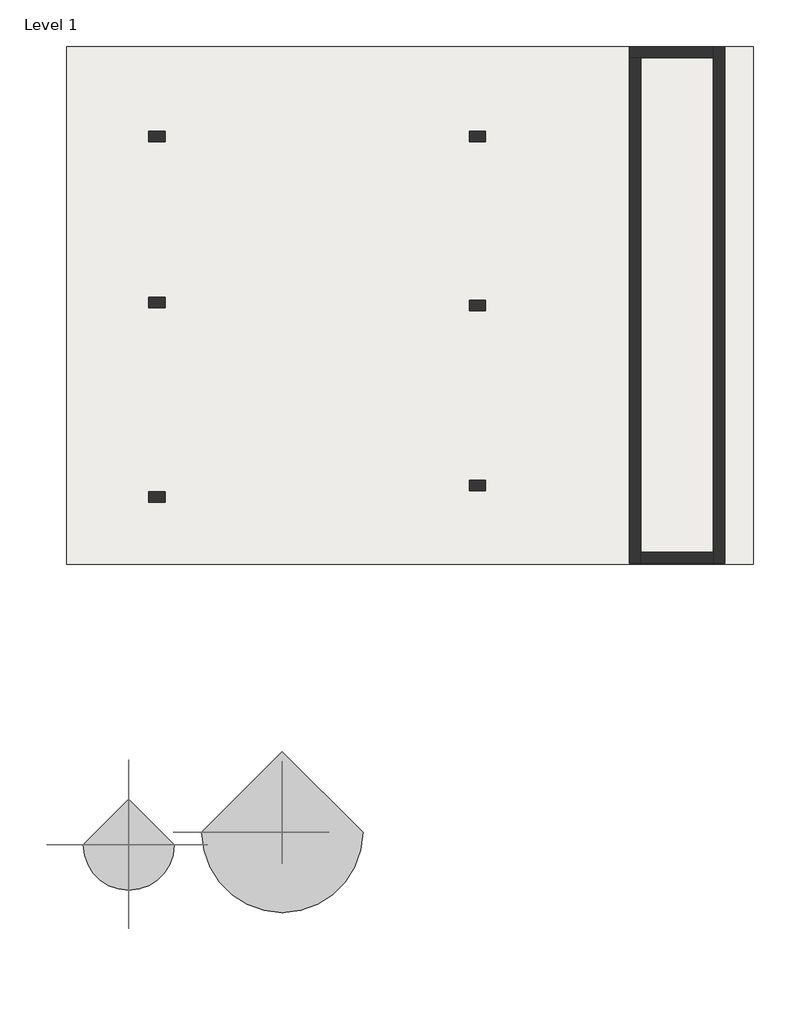
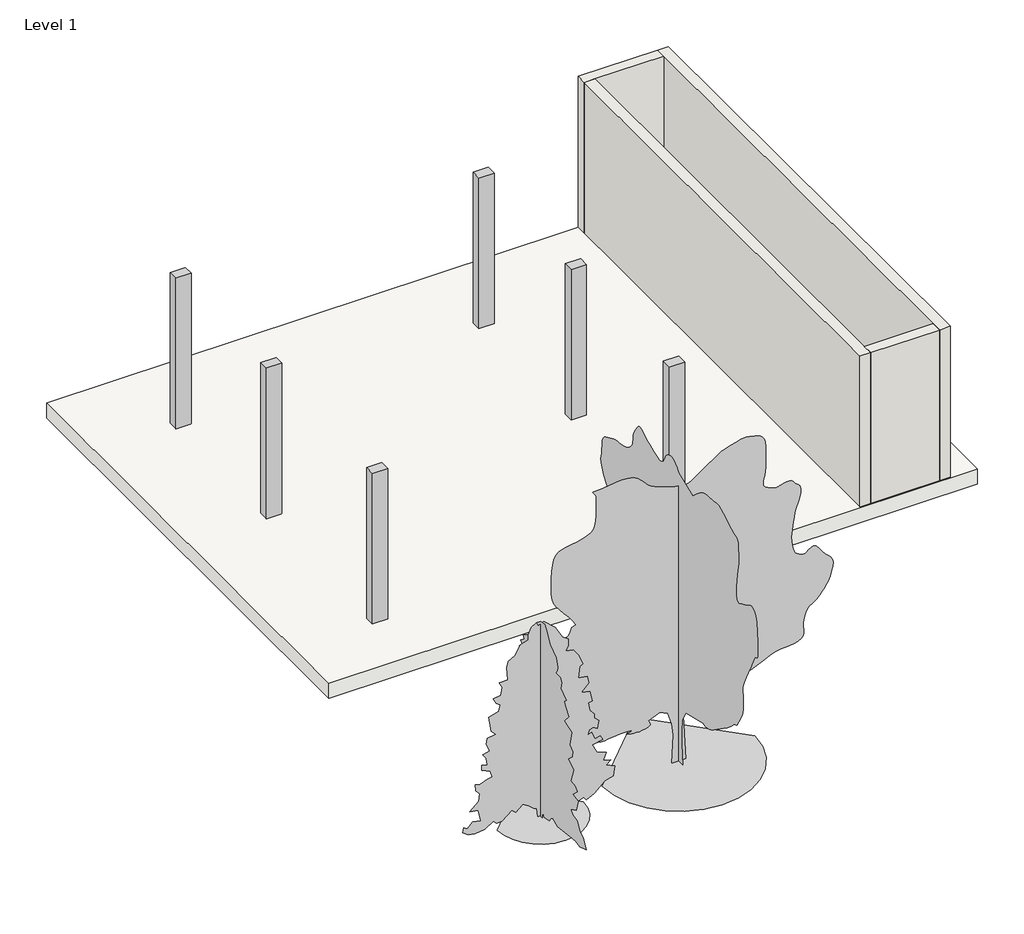
# One storey: 6 columns, 4 walls, 2 geographic elements, 1 slab.
"""IFC4 building model written with IfcOpenShell, lengths in millimetres."""

from ifc_helpers import new_model, si_unit, frame, origin, origin_with_axes, place, context, project, spatial, polyline, outline, extrude, faceted_brep, transform, mapped, element, save
from components import wood_timber_column_8_x_12_245a0583, rpc_tree_conifer_97aab292, rpc_tree_deciduous_american_beech_20_b3c041c8

model = new_model("IFC4")

# Units and contexts
model_context = context("Model", 3, world=origin())
ifc_project = project(units=[si_unit("LENGTHUNIT", "METRE", prefix="MILLI")], contexts=[model_context])

# Site, building, storey
site = spatial("IfcSite", under=ifc_project)
building = spatial("IfcBuilding", under=site)
storey = spatial("IfcBuildingStorey", under=building, Name="Level 1", Elevation=0.0)

# Columns
placement = place(None, origin())
wood_timber_column_8_x_12_shape = wood_timber_column_8_x_12_245a0583(model_context)
element("IfcColumn", 1, ObjectType="Wood Timber Column : 8 x 12", at=placement, inside=storey, context=model_context, shape_type="MappedRepresentation", body=[
    mapped(wood_timber_column_8_x_12_shape, transform((-15839.6169582, -7474.3117616, 0.0), x_axis=(0.0, 1.0000000000000002, 0.0), y_axis=(-1.0000000000000002, 0.0, 0.0), z_axis=(0.0, 0.0, 1.0))),
])
element("IfcColumn", 2, ObjectType="Wood Timber Column : 8 x 12", at=placement, inside=storey, context=model_context, shape_type="MappedRepresentation", body=[
    mapped(wood_timber_column_8_x_12_shape, transform((-10048.4169582, -7271.1117616, 0.0), x_axis=(0.0, 1.0000000000000002, 0.0), y_axis=(-1.0000000000000002, 0.0, 0.0), z_axis=(0.0, 0.0, 1.0))),
])
element("IfcColumn", 3, ObjectType="Wood Timber Column : 8 x 12", at=placement, inside=storey, context=model_context, shape_type="MappedRepresentation", body=[
    mapped(wood_timber_column_8_x_12_shape, transform((-10048.4169582, -4019.9117616, 0.0), x_axis=(0.0, 1.0000000000000002, 0.0), y_axis=(-1.0000000000000002, 0.0, 0.0), z_axis=(0.0, 0.0, 1.0))),
])
element("IfcColumn", 4, ObjectType="Wood Timber Column : 8 x 12", at=placement, inside=storey, context=model_context, shape_type="MappedRepresentation", body=[
    mapped(wood_timber_column_8_x_12_shape, transform((-15839.6169582, -3969.1117616, 0.0), x_axis=(0.0, 1.0000000000000002, 0.0), y_axis=(-1.0000000000000002, 0.0, 0.0), z_axis=(0.0, 0.0, 1.0))),
])
element("IfcColumn", 5, ObjectType="Wood Timber Column : 8 x 12", at=placement, inside=storey, context=model_context, shape_type="MappedRepresentation", body=[
    mapped(wood_timber_column_8_x_12_shape, transform((-15839.6169582, -971.9117616, 0.0), x_axis=(0.0, 1.0000000000000002, 0.0), y_axis=(-1.0000000000000002, 0.0, 0.0), z_axis=(0.0, 0.0, 1.0))),
])
element("IfcColumn", 6, ObjectType="Wood Timber Column : 8 x 12", at=placement, inside=storey, context=model_context, shape_type="MappedRepresentation", body=[
    mapped(wood_timber_column_8_x_12_shape, transform((-10048.4169582, -971.9117616, 0.0), x_axis=(0.0, 1.0000000000000002, 0.0), y_axis=(-1.0000000000000002, 0.0, 0.0), z_axis=(0.0, 0.0, 1.0))),
])

# Geographic elements
rpc_tree_conifer_shape = rpc_tree_conifer_97aab292(model_context)
element("IfcGeographicElement", 7, ObjectType="RPC Tree - Conifer", at=placement, inside=storey, context=model_context, shape_type="MappedRepresentation", body=[
    mapped(rpc_tree_conifer_shape, transform((-16347.8136293, -13754.4617616, 0.0), x_axis=(1.0, 0.0, 0.0), y_axis=(0.0, 1.0, 0.0), z_axis=(0.0, 0.0, 1.0))),
])
rpc_tree_deciduous_american_beech_20_shape = rpc_tree_deciduous_american_beech_20_b3c041c8(model_context)
element("IfcGeographicElement", 8, ObjectType="RPC Tree - Deciduous : American Beech - 20'", at=placement, inside=storey, context=model_context, shape_type="MappedRepresentation", body=[
    mapped(rpc_tree_deciduous_american_beech_20_shape, transform((-13574.3729387, -13525.8617616, 0.0), x_axis=(1.0, 0.0, 0.0), y_axis=(0.0, 1.0, 0.0), z_axis=(0.0, 0.0, 1.0))),
])

# Slab
element("IfcSlab", 9, ObjectType="Generic - 12\" 3", at=placement, inside=storey, context=model_context, shape_type="SweptSolid", body=[
    extrude(outline(polyline([(-5070.0169582, 653.6882384), (-5070.0169582, -8693.5117616), (-17465.2169582, -8693.5117616), (-17465.2169582, 653.6882384), (-5070.0169582, 653.6882384)])), frame((0.0, 0.0, -304.8), z_axis=(0.0, 0.0, 1.0), x_axis=(1.0, 0.0, 0.0)), (0.0, 0.0, 1.0), 304.8),
])

# Walls
element("IfcWall", 10, ObjectType="Generic - 8\" 3", at=placement, inside=storey, context=model_context, shape_type="Brep", body=[
    faceted_brep([(-5784.3919582, 653.6882384, 0.0), (-5784.3919582, 450.4882384, 0.0), (-5784.3919582, -8471.2617616, 0.0), (-5784.3919582, -8674.4617616, 0.0), (-5784.3919582, -8674.4617616, 3048.0), (-5784.3919582, -8471.2617616, 3048.0), (-5784.3919582, 450.4882384, 3048.0), (-5784.3919582, 653.6882384, 3048.0), (-5581.1919582, 653.6882384, 0.0), (-5581.1919582, 653.6882384, 3048.0), (-5581.1919582, -8674.4617616, 3048.0), (-5581.1919582, -8674.4617616, 0.0)], [[[0, 1, 2, 3, 4, 5, 6, 7]], [[8, 9, 10, 11]], [[3, 2, 1, 0, 8, 11]], [[7, 6, 5, 4, 10, 9]], [[0, 7, 9, 8]], [[4, 3, 11, 10]]]),
])
element("IfcWall", 11, ObjectType="Generic - 8\" 3", at=placement, inside=storey, context=model_context, shape_type="Brep", body=[
    faceted_brep([(-5784.3919582, 653.6882384, 0.0), (-7305.2169582, 653.6882384, 0.0), (-7305.2169582, 653.6882384, 3048.0), (-5784.3919582, 653.6882384, 3048.0), (-5784.3919582, 450.4882384, 0.0), (-5784.3919582, 450.4882384, 3048.0), (-7102.0169582, 450.4882384, 3048.0), (-7305.2169582, 450.4882384, 3048.0), (-7305.2169582, 450.4882384, 0.0), (-7102.0169582, 450.4882384, 0.0)], [[[0, 1, 2, 3]], [[4, 5, 6, 7, 8, 9]], [[1, 0, 4, 9, 8]], [[3, 2, 7, 6, 5]], [[0, 3, 5, 4]], [[2, 1, 8, 7]]]),
])
element("IfcWall", 12, ObjectType="Generic - 8\" 3", at=placement, inside=storey, context=model_context, shape_type="Brep", body=[
    faceted_brep([(-7305.2169582, 450.4882384, 0.0), (-7305.2169582, -8674.4617616, 0.0), (-7305.2169582, -8674.4617616, 3048.0), (-7305.2169582, 450.4882384, 3048.0), (-7102.0169582, 450.4882384, 0.0), (-7102.0169582, 450.4882384, 3048.0), (-7102.0169582, -8471.2617616, 3048.0), (-7102.0169582, -8674.4617616, 3048.0), (-7102.0169582, -8674.4617616, 0.0), (-7102.0169582, -8471.2617616, 0.0)], [[[0, 1, 2, 3]], [[4, 5, 6, 7, 8, 9]], [[1, 0, 4, 9, 8]], [[3, 2, 7, 6, 5]], [[0, 3, 5, 4]], [[2, 1, 8, 7]]]),
])
element("IfcWall", 13, ObjectType="Generic - 8\" 3", at=placement, inside=storey, context=model_context, shape_type="SweptSolid", body=[
    extrude(outline(polyline([(-5784.3919582, -8674.4617616), (-7102.0169582, -8674.4617616), (-7102.0169582, -8471.2617616), (-5784.3919582, -8471.2617616), (-5784.3919582, -8674.4617616)])), origin_with_axes(), (0.0, 0.0, 1.0), 3048.0),
])

save(model, "model.ifc")

# Revit data of these elements
# Type "Wood Timber Column : 8 x 12"
#   Assembly Code = "B1010200"
#   Depth = 0' - 11 1/2"
#   Width = 0' - 7 1/2"
#   Material = Rigid insulation
# Type "RPC Tree - Conifer"
#   built-in parameter 1005198 = "{2, 15},{39, RPC-16-G0M4-N9PX-U6TN-C000-ST1L-LVER-AU},{1, 0},{1, 0},{2, 13},{1, 8},{5, Color},{1, 0},{1, 0},{3, 0.8},{3, 0.8},{3, 0.8},{1, 8},{7, BBoxMin},{1, 0},{1, 0},{1, 0},{1, 0},{1, 0},{1, 8},{7, BBoxMax},{1, 0},{1, 0},{1, 0},{1, 0},{1, 0},{2, 11},{9, RPCTypeId},{1, 0},{1, 0},{39, RPC-16-G0M4-N9PX-U6TN-C000-ST1L-LVER-AU},{1, 6},{14, RPCPlantHeight},{1, 0},{1, 0},{2, 13},{2, 11},{7, keyword},{1, 0},{1, 0},{34, :RPCs:Trees [General]:Geometry:RPC},{2, 11},{8, category},{1, 0},{1, 0},{15, Trees [General]},{2, 11},{12, LocalizedUID},{1, 0},{1, 0},{15, Colorado Spruce},{2, 14},{6, Height},{1, 0},{1, 0},{2, 13},{1, 2},{16, Cast Reflections},{1, 0},{1, 0},{1, 0},{1, 2},{12, Cast Shadows},{1, 0},{1, 0},{1, 1},{1, 2},{9, Lock View},{1, 0},{1, 0},{1, 0},{1, 4},{5, ViewC},{1, 0},{1, 0},{1, 0},{21, assetlibrary_base.fbx},{1, 5},"
#   built-in parameter 1005195 = "RPC-16-G0M4-N9PX-U6TN-C000-ST1L-LVER-AU"
#   Assembly Code = "G2050500"
#   Height = 13' - 0"
#   Description = (empty or 0)
#   Default Elevation = 0
# Type "RPC Tree - Deciduous : American Beech - 20'"
#   built-in parameter 1005198 = "{2, 15},{39, RPC-16-G1GQ-43Q0-7NP3-0000-ST1L-LVER-AU},{1, 0},{1, 0},{2, 13},{1, 8},{5, Color},{1, 0},{1, 0},{3, 0.8},{3, 0.8},{3, 0.8},{1, 8},{7, BBoxMin},{1, 0},{1, 0},{1, 0},{1, 0},{1, 0},{1, 8},{7, BBoxMax},{1, 0},{1, 0},{1, 0},{1, 0},{1, 0},{2, 11},{9, RPCTypeId},{1, 0},{1, 0},{39, RPC-16-G1GQ-43Q0-7NP3-0000-ST1L-LVER-AU},{1, 6},{14, RPCPlantHeight},{1, 0},{1, 0},{2, 20},{2, 11},{7, keyword},{1, 0},{1, 0},{34, :RPCs:Trees [General]:Geometry:RPC},{2, 11},{8, category},{1, 0},{1, 0},{15, Trees [General]},{2, 11},{12, LocalizedUID},{1, 0},{1, 0},{14, American Beech},{2, 14},{6, Height},{1, 0},{1, 0},{2, 20},{1, 2},{16, Cast Reflections},{1, 0},{1, 0},{1, 0},{1, 2},{12, Cast Shadows},{1, 0},{1, 0},{1, 1},{1, 2},{9, Lock View},{1, 0},{1, 0},{1, 0},{1, 4},{5, ViewC},{1, 0},{1, 0},{1, 0},{21, assetlibrary_base.fbx},{1, 5},"
#   built-in parameter 1005195 = "RPC-16-G1GQ-43Q0-7NP3-0000-ST1L-LVER-AU"
#   Type Comments = "American Beech"
#   Assembly Code = "G2050500"
#   Height = 20' - 0"
#   Default Elevation = 0
# Type "Generic - 12\" 3"
#   Assembly Code = "B1010"
#   Function = 0
#   Layers, outside or top first: 1' - 0" "Rigid insulation" (function 1)
# Type "Generic - 8\" 3"
#   Assembly Code = "B2010"
#   Layers, outside or top first: 0' - 8" "EIFS, Exterior Insulation" (function 1)
# Elements 1, 2, 3, 4, 5, 6 (IfcColumn, "Wood Timber Column : 8 x 12")
#   Phase Created = New Construction
#   Materials on its faces: "Rigid insulation"
# Element 7 (IfcGeographicElement, "RPC Tree - Conifer")
#   Phase Created = New Construction
# Element 8 (IfcGeographicElement, "RPC Tree - Deciduous : American Beech - 20'")
#   Phase Created = New Construction
# Element 9 (IfcSlab, "Generic - 12\" 3")
#   Height Offset From Level = 0' - 0"
#   Phase Created = New Construction
#   Materials on its faces: "Rigid insulation"
# Elements 10, 11, 12, 13 (IfcWall, "Generic - 8\" 3")
#   Top Offset = 0' - 0"
#   Base Offset = 0' - 0"
#   Unconnected Height = 10' - 0"
#   wall height = 10' - 0"
#   Phase Created = New Construction
#   Base Constraint = Level 1
#   Materials on its faces: "EIFS, Exterior Insulation"
# Materials
#   "Rigid insulation": class "Generic", colour RGB 127 127 127, transparency 0, Description = "Rigid foam insulation board", Cost = 0
#   "EIFS, Exterior Insulation": class "Generic", colour RGB 127 127 127, transparency 0, Description = "EIFS - Exterior Insulation", Cost = 0
